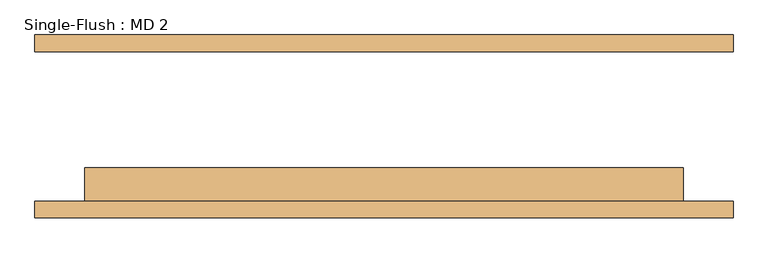
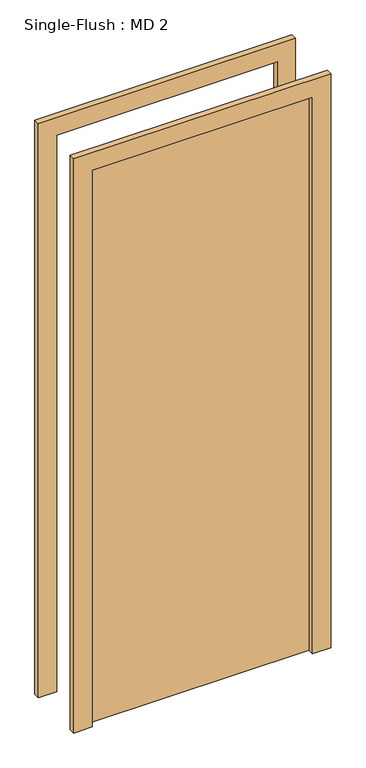
"""IFC4 building model written with IfcOpenShell, lengths in millimetres: door geometry, Single-Flush : MD 2."""

from ifc_helpers import new_model, si_unit, frame, origin, origin_with_axes, place, context, project, spatial, polyline, outline, extrude, source, transform, mapped, element, save


def single_flush_md_2_ea82e2eb(model_context):
    return source(origin(), model_context, "Body", "SweptSolid", [
        extrude(outline(polyline([(2514.6, -533.4), (0.0, -533.4), (0.0, -457.2), (2438.4, -457.2), (2438.4, 457.2), (0.0, 457.2), (0.0, 533.4), (2514.6, 533.4), (2514.6, -533.4)])), frame((0.0, -139.7, 0.0), z_axis=(0.0, 1.0, 0.0), x_axis=(0.0, 0.0, 1.0)), (0.0, 0.0, 1.0), 25.4),
        extrude(outline(polyline([(2514.6, 533.4), (2514.6, -533.4), (0.0, -533.4), (0.0, -457.2), (2438.4, -457.2), (2438.4, 457.2), (0.0, 457.2), (0.0, 533.4), (2514.6, 533.4)])), frame((0.0, 114.3, 0.0), z_axis=(0.0, 1.0, 0.0), x_axis=(0.0, 0.0, 1.0)), (0.0, 0.0, 1.0), 25.4),
        extrude(outline(polyline([(457.2, -63.5), (457.2, -114.3), (-457.2, -114.3), (-457.2, -63.5), (457.2, -63.5)])), origin_with_axes(), (0.0, 0.0, 1.0), 2438.4),
    ])


if __name__ == "__main__":
    model = new_model("IFC4")
    model_context = context("Model", 3, world=origin())
    ifc_project = project(units=[si_unit("LENGTHUNIT", "METRE", prefix="MILLI")], contexts=[model_context])
    site = spatial("IfcSite", under=ifc_project)
    building = spatial("IfcBuilding", under=site)
    placement = place(None, origin())
    single_flush_md_2_shape = single_flush_md_2_ea82e2eb(model_context)
    element("IfcDoor", 1, ObjectType="Single-Flush : MD 2", at=placement, inside=building, context=model_context, shape_type="MappedRepresentation", body=[
        mapped(single_flush_md_2_shape, transform((0.0, 0.0, 0.0), x_axis=(1.0, 0.0, 0.0), y_axis=(0.0, 1.0, 0.0), z_axis=(0.0, 0.0, 1.0))),
    ])
    save(model, "model.ifc")

# Revit data of these elements
# Type "Single-Flush : MD 2"
#   Type Mark = "11"
#   Construction Type Id = "MDOOR"
#   Assembly Code = "C1020"
#   Analytic Construction = "Metal"
#   Thickness = 0' - 2"
#   Heat Transfer Coefficient (U) = 0.651978 BTU/(h·ft²·°F)
#   Height = 8' - 0"
#   Trim Projection Ext = 0' - 1"
#   Trim Projection Int = 0' - 1"
#   Trim Width = 0' - 3"
#   Width = 3' - 0"
#   Define Thermal Properties by = 1
#   Door Material = Door - Panel
#   Frame Material = Door - Frame
#   Visual Light Transmittance = 0
#   Solar Heat Gain Coefficient = 0
#   Function = (empty or 0)
#   Wall Closure = (empty or 0)
# Element 1 (IfcDoor, "Single-Flush : MD 2")
#   Materials on its faces: "Door - Frame", "Door - Panel"
# Materials
#   "Door - Panel": class "Wood", colour RGB 210 159 95, transparency 0, Cost = 0
#   "Door - Frame": colour RGB 118 70 51, transparency 0, Cost = 0
